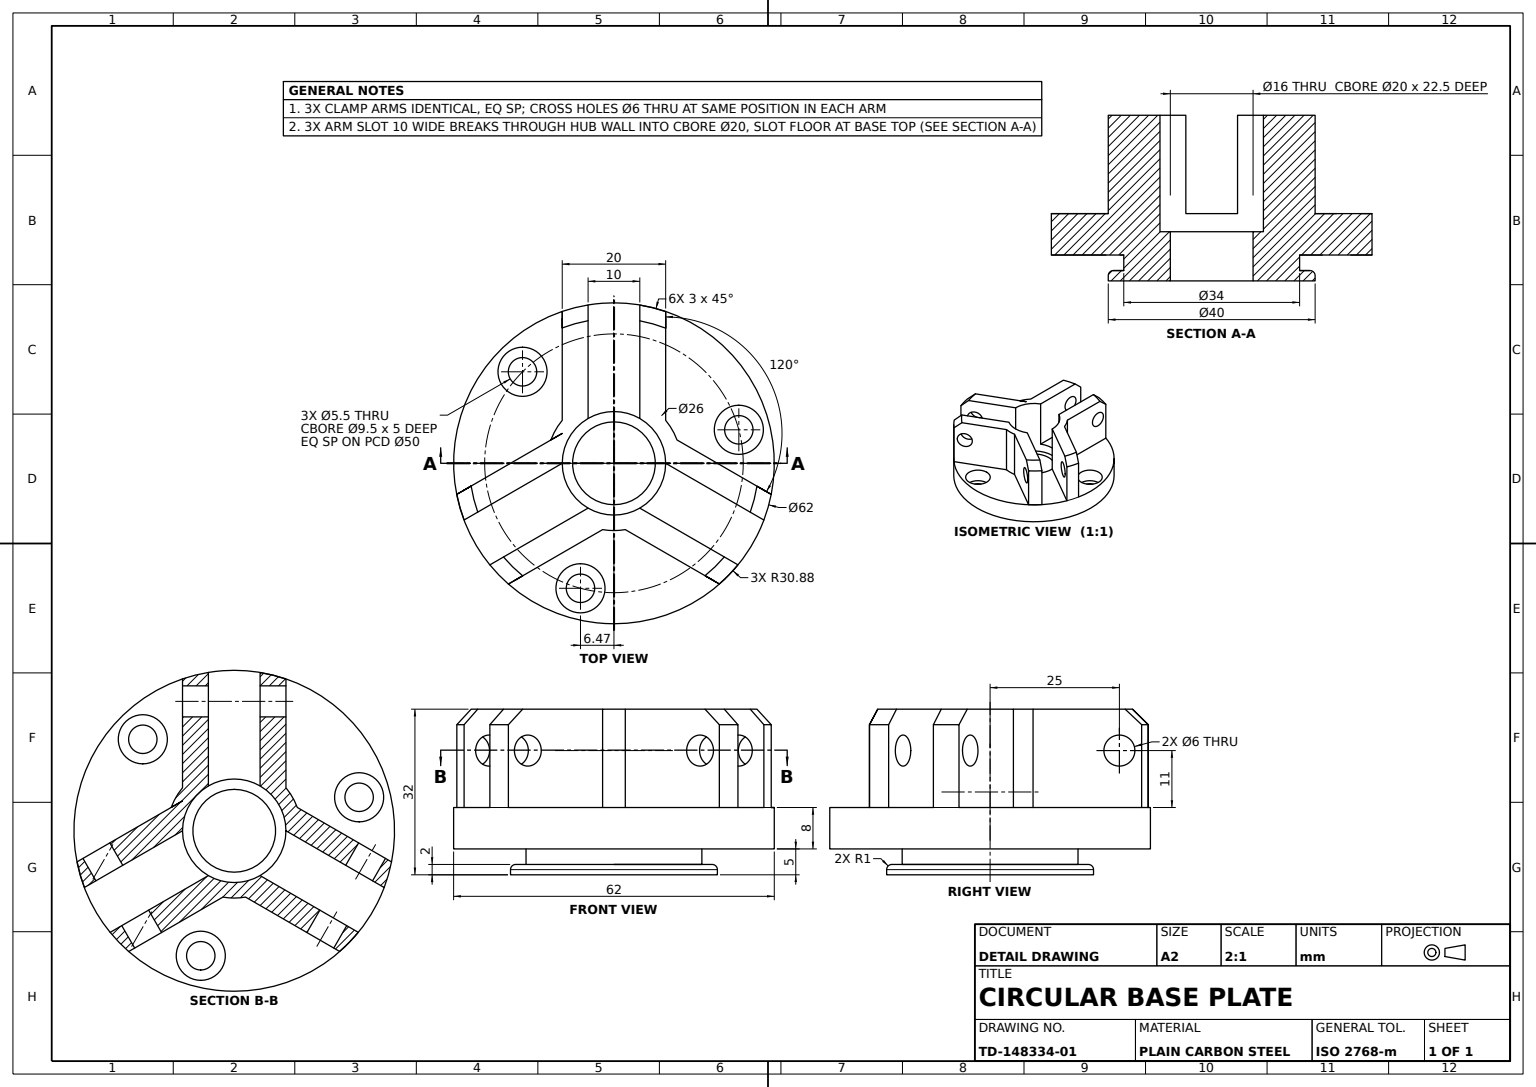
from build123d import *

# Parameters (mm, degrees)
BASE_DISC_SKETCH_R             = 31
BASE_DISC_62_DEPTH             = 13
CLAMP_ARMS_DEPTH               = 19
CENTRE_BORE_SKETCH_R           = 10
CENTRE_BORE_DEPTH              = 22.5
CENTRE_HUB_DEPTH               = 20
MOUNTING_COUNTERBORES_SKETCH_R = 4.75
MOUNTING_COUNTERBORES_DEPTH    = 5
ARM_CROSS_HOLE_1_SKETCH_R      = 3
ARM_CROSS_HOLE_1_DEPTH         = 32
ARM_CROSS_HOLE_2_SKETCH_R      = 3
ARM_CROSS_HOLE_2_DEPTH         = 32
ARM_CROSS_HOLE_3_SKETCH_R      = 3
ARM_CROSS_HOLE_3_DEPTH         = 32
MOUNTING_HOLES_SKETCH_R        = 2.75
MOUNTING_HOLES_3X_DEPTH        = 32
CENTRE_THROUGH_BORE_SKETCH_R   = 8
CENTRE_THROUGH_BORE_DEPTH      = 32
ARM_CHAMFER_1_SIZE             = 3
ARM_CHAMFER_2_SIZE             = 3
ARM_CHAMFER_3_SIZE             = 3
ARM_CHAMFER_4_SIZE             = 3
ARM_CHAMFER_5_SIZE             = 3
ARM_CHAMFER_6_SIZE             = 3
BOTTOM_RECESS_SKETCH_R         = 31
BOTTOM_RECESS_DEPTH            = 5
RECESS_RING_SKETCH_R           = 17
RECESS_RING_DEPTH              = 3
LOCATING_LIP_SKETCH_R          = 20
LOCATING_LIP_DEPTH             = 2
LOCATING_LIP_FILLET_R1_R       = 1
LIP_BORE_SKETCH_R              = 8
LIP_BORE_DEPTH                 = 19


with BuildPart() as part:
    # Base Disc Sketch → Base Disc Ø62 (new body)
    with BuildSketch(Plane(origin=(0, 0, 0), x_dir=(1, 0, 0), z_dir=(0, 1, 0))):
        with Locations(Location((0, 0, 0), (0, 0, 90))):
            Circle(BASE_DISC_SKETCH_R)
    extrude(amount=BASE_DISC_62_DEPTH)

    # Clamp Arms Sketch → Clamp Arms (add)
    with BuildSketch(Plane(origin=(0, 13, 0), x_dir=(1, 0, 0), z_dir=(0, 1, 0))):
        with BuildLine():
            Line((10, 29.304386049), (10, 5.773502692))
            Line((10, 5.773502692), (30.411611519, -6.011146713))
            ThreePointArc((30.411611519, -6.011146713), (29.804874358, -8.517522175), (28.991130921, -10.96453455))
            Line((28.991130921, -10.96453455), (5, 2.886751346))
            Line((5, 2.886751346), (5, 30.570907429))
            ThreePointArc((5, 30.570907429), (7.526489622, 30.042223032), (10, 29.304386049))
        make_face()
        with BuildLine():
            Line((-10, 29.342801502), (-10, 5.773502692))
            Line((-10, 5.773502692), (-30.378342761, -5.991938987))
            ThreePointArc((-30.378342761, -5.991938987), (-29.780573143, -8.502980302), (-28.97518245, -10.955326696))
            Line((-28.97518245, -10.955326696), (-5, 2.886751346))
            Line((-5, 2.886751346), (-5, 30.589323137))
            ThreePointArc((-5, 30.589323137), (-7.526046598, 30.070539438), (-10, 29.342801502))
        make_face()
        with BuildLine():
            Line((23.97518245, -19.615580733), (0, -5.773502692))
            Line((0, -5.773502692), (-23.991130921, -19.624788587))
            ThreePointArc((-23.991130921, -19.624788587), (-22.27882776, -21.553017263), (-20.411611519, -23.331654789))
            Line((-20.411611519, -23.331654789), (0, -11.547005384))
            Line((0, -11.547005384), (20.378342761, -23.312447062))
            ThreePointArc((20.378342761, -23.312447062), (22.254083521, -21.53924273), (23.97518245, -19.615580733))
        make_face()
    extrude(amount=CLAMP_ARMS_DEPTH)

    # Centre Bore Sketch → Centre Bore (cut)
    with BuildSketch(Plane(origin=(0, 32, 0), x_dir=(1, 0, 0), z_dir=(0, 1, 0))):
        with Locations(Location((0, 0, 0), (0, 0, 270))):
            Circle(CENTRE_BORE_SKETCH_R)
    extrude(amount=-CENTRE_BORE_DEPTH, mode=Mode.SUBTRACT)

    # Centre Hub Sketch → Centre Hub (add)
    with BuildSketch(Plane(origin=(0, 32, 0), x_dir=(1, 0, 0), z_dir=(0, 1, 0))):
        with BuildLine():
            Line((-10, 8.306623863), (-10, 5.773502692))
            Line((-10, 5.773502692), (-12.188322207, 4.521592837))
            ThreePointArc((-12.188322207, 4.521592837), (-11.254422489, 6.506763746), (-10, 8.306623863))
        make_face()
        with BuildLine():
            Line((10, 8.306623863), (10, 5.773502692))
            Line((10, 5.773502692), (12.193747285, 4.506942106))
            ThreePointArc((12.193747285, 4.506942106), (11.258330249, 6.5), (10, 8.306623863))
        make_face()
        with BuildLine():
            Line((-2.193747285, -12.813565969), (0, -11.547005384))
            Line((0, -11.547005384), (2.193747285, -12.813565969))
            ThreePointArc((2.193747285, -12.813565969), (0, -13), (-2.193747285, -12.813565969))
        make_face()
    extrude(amount=-CENTRE_HUB_DEPTH)

    # Mounting Counterbores Sketch → Mounting Counterbores (cut)
    with BuildSketch(Plane(origin=(0, 13, 0), x_dir=(1, 0, 0), z_dir=(0, 1, 0))):
        with Locations(Location((-6.470476128, -24.148145657, 0), (0, 0, 270))):
            Circle(MOUNTING_COUNTERBORES_SKETCH_R)
        with Locations(Location((24.148145657, 6.470476128, 0), (0, 0, 270))):
            Circle(MOUNTING_COUNTERBORES_SKETCH_R)
        with Locations(Location((-17.67766953, 17.67766953, 0), (0, 0, 270))):
            Circle(MOUNTING_COUNTERBORES_SKETCH_R)
    extrude(amount=-MOUNTING_COUNTERBORES_DEPTH, mode=Mode.SUBTRACT)

    # Arm Cross Hole 1 Sketch → Arm Cross Hole 1 (cut)
    with BuildSketch(Plane.ZY.offset(10)):
        with Locations((-25, 24)):
            Circle(ARM_CROSS_HOLE_1_SKETCH_R)
    extrude(amount=-ARM_CROSS_HOLE_1_DEPTH, mode=Mode.SUBTRACT)

    # Arm Cross Hole 2 Sketch → Arm Cross Hole 2 (cut)
    with BuildSketch(Plane(origin=(5, 0, -8.660254038), x_dir=(-0.8660254037844363, 0, -0.5000000000000043), z_dir=(0.5000000000000042, 0, -0.8660254037844362))):
        with Locations((-25, 24)):
            Circle(ARM_CROSS_HOLE_2_SKETCH_R)
    extrude(amount=-ARM_CROSS_HOLE_2_DEPTH, mode=Mode.SUBTRACT)

    # Arm Cross Hole 3 Sketch → Arm Cross Hole 3 (cut)
    with BuildSketch(Plane(origin=(5, 0, 8.660254038), x_dir=(0.8660254037844433, 0, -0.4999999999999921), z_dir=(0.49999999999999206, 0, 0.8660254037844431))):
        with Locations((-25, 24)):
            Circle(ARM_CROSS_HOLE_3_SKETCH_R)
    extrude(amount=-ARM_CROSS_HOLE_3_DEPTH, mode=Mode.SUBTRACT)

    # Mounting Holes Sketch → Mounting Holes 3x (cut)
    with BuildSketch(Plane(origin=(0, 8, 0), x_dir=(1, 0, 0), z_dir=(0, 1, 0))):
        with Locations(Location((-17.67766953, 17.67766953, 0), (0, 0, 270))):
            Circle(MOUNTING_HOLES_SKETCH_R)
        with Locations(Location((24.148145657, 6.470476128, 0), (0, 0, 270))):
            Circle(MOUNTING_HOLES_SKETCH_R)
        with Locations(Location((-6.470476128, -24.148145657, 0), (0, 0, 270))):
            Circle(MOUNTING_HOLES_SKETCH_R)
    extrude(amount=-MOUNTING_HOLES_3X_DEPTH, mode=Mode.SUBTRACT)

    # Centre Through Bore Sketch → Centre Through Bore (cut)
    with BuildSketch(Plane(origin=(0, 9.5, 0), x_dir=(1, 0, 0), z_dir=(0, 1, 0))):
        with Locations(Location((0, 0, 0), (0, 0, 270))):
            Circle(CENTRE_THROUGH_BORE_SKETCH_R)
    extrude(amount=-CENTRE_THROUGH_BORE_DEPTH, mode=Mode.SUBTRACT)

    # Arm Chamfer 1
    arm_chamfer_1_edges = [part.edges().sort_by_distance(p)[0] for p in [
        (-29.780573143, 32, 8.502980302),
    ]]
    chamfer(arm_chamfer_1_edges, length=ARM_CHAMFER_1_SIZE)

    # Arm Chamfer 2
    arm_chamfer_2_edges = [part.edges().sort_by_distance(p)[0] for p in [
        (-22.27882776, 32, 21.553017263),
    ]]
    chamfer(arm_chamfer_2_edges, length=ARM_CHAMFER_2_SIZE)

    # Arm Chamfer 3
    arm_chamfer_3_edges = [part.edges().sort_by_distance(p)[0] for p in [
        (22.254083521, 32, 21.53924273),
    ]]
    chamfer(arm_chamfer_3_edges, length=ARM_CHAMFER_3_SIZE)

    # Arm Chamfer 4
    arm_chamfer_4_edges = [part.edges().sort_by_distance(p)[0] for p in [
        (29.804874358, 32, 8.517522175),
    ]]
    chamfer(arm_chamfer_4_edges, length=ARM_CHAMFER_4_SIZE)

    # Arm Chamfer 5
    arm_chamfer_5_edges = [part.edges().sort_by_distance(p)[0] for p in [
        (7.526489622, 32, -30.042223032),
    ]]
    chamfer(arm_chamfer_5_edges, length=ARM_CHAMFER_5_SIZE)

    # Arm Chamfer 6
    arm_chamfer_6_edges = [part.edges().sort_by_distance(p)[0] for p in [
        (-7.526046598, 32, -30.070539438),
    ]]
    chamfer(arm_chamfer_6_edges, length=ARM_CHAMFER_6_SIZE)

    # Bottom Recess Sketch → Bottom Recess (cut)
    with BuildSketch(Plane.XZ):
        with Locations(Location((0, 0, 0), (0, 0, 270))):
            Circle(BOTTOM_RECESS_SKETCH_R)
    extrude(amount=-BOTTOM_RECESS_DEPTH, mode=Mode.SUBTRACT)

    # Recess Ring Sketch → Recess Ring (add)
    with BuildSketch(Plane.XZ.offset(-5)):
        with Locations(Location((0, 0, 0), (0, 0, 270))):
            Circle(RECESS_RING_SKETCH_R)
    extrude(amount=RECESS_RING_DEPTH)

    # Locating Lip Sketch → Locating Lip (add)
    with BuildSketch(Plane.XZ.offset(-2)):
        with Locations(Location((0, 0, 0), (0, 0, 270))):
            Circle(LOCATING_LIP_SKETCH_R)
    extrude(amount=LOCATING_LIP_DEPTH)

    # Locating Lip Fillet R1
    locating_lip_fillet_r1_edges = [part.edges().sort_by_distance(p)[0] for p in [
        (0, 2, 20),
    ]]
    fillet(locating_lip_fillet_r1_edges, radius=LOCATING_LIP_FILLET_R1_R)

    # Lip Bore Sketch → Lip Bore (cut)
    with BuildSketch(Plane(origin=(0, 5, 0), x_dir=(1, 0, 0), z_dir=(0, 1, 0))):
        with Locations(Location((0, 0, 0), (0, 0, 270))):
            Circle(LIP_BORE_SKETCH_R)
    extrude(amount=-LIP_BORE_DEPTH, mode=Mode.SUBTRACT)


solid = part.part
